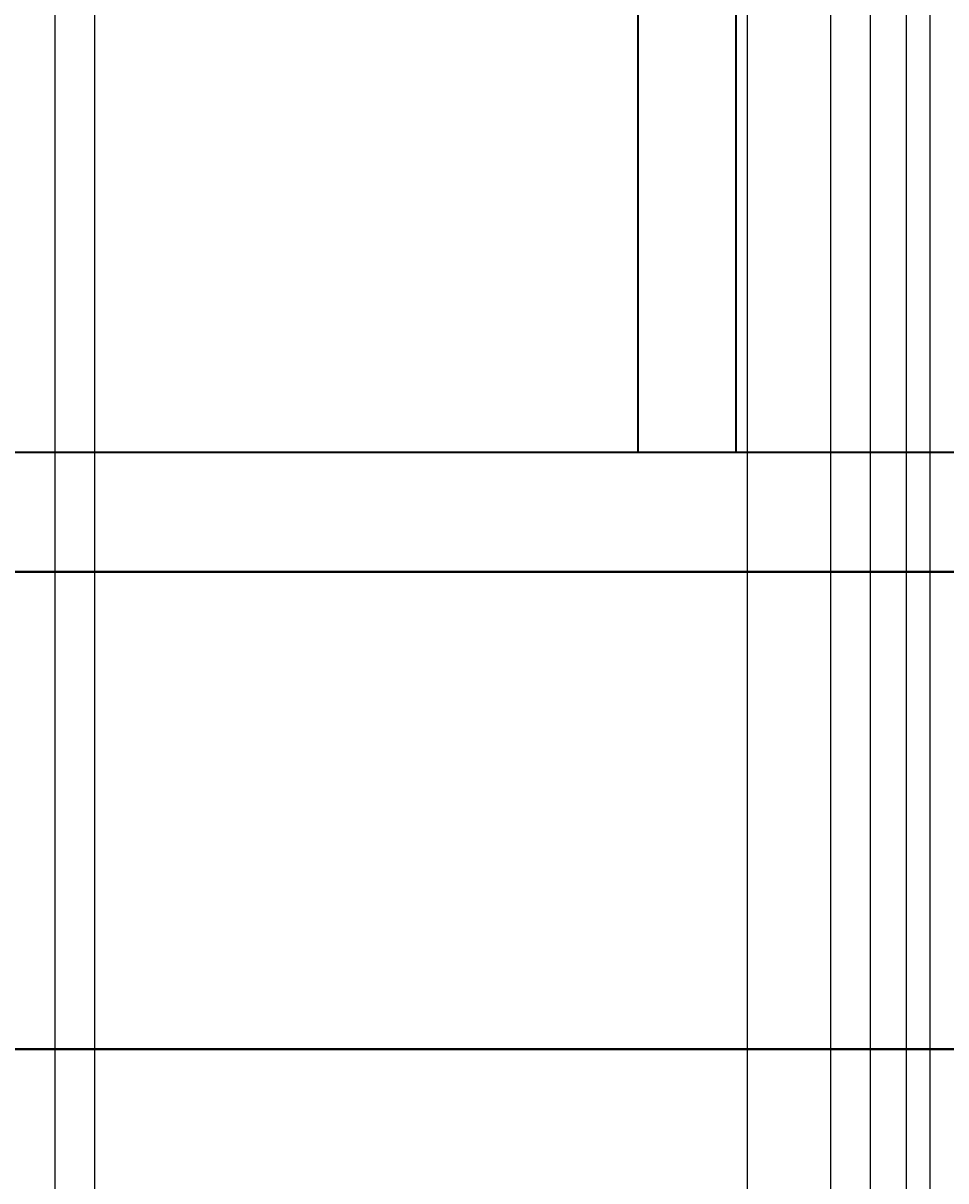
# Model space of a CAD drawing. Units: inches. Extents: x -6 to 289, y -8 to 323.
# Tile 52 of 107: x 146 to 169, y 124 to 153. Entities that reach past the tile are written whole.
import ezdxf

# ---------------------------------------------------------------- set-up
doc = ezdxf.new("R2010")
doc.units = ezdxf.units.IN
doc.header["$MEASUREMENT"] = 0
doc.layers.add('A-ANNO-DIMS', color=2, linetype='Continuous', lineweight=18)
doc.layers.add('A-ELEV', color=7, linetype='Continuous', lineweight=35)
doc.styles.get("Standard").update_dxf_attribs({"font": 'arial.ttf'})
doc.dimstyles.get("Standard").update_dxf_attribs({"dimtxt": 0.18, "dimasz": 0.18, "dimexe": 0.18, "dimexo": 0.0625, "dimgap": 0.09, "dimtad": 0, "dimtih": 1, "dimtoh": 1, "dimdec": 4, "dimzin": 0, "dimdsep": 46, "dimtxsty": 'Standard', "dimcen": 0.09, "dimadec": 0, "dimazin": 0, "dimtfac": 1, "dimtdec": 4, "dimtofl": 0, "dimtmove": 0, "dimatfit": 3, "dimfxl": 1, "dimtolj": 1, "dimtzin": 0, "dimarcsym": 0})

# ---------------------------------------------------------------- blocks, each defined once
blk = doc.blocks.new('*D24')
at = {"layer": 'A-ANNO-DIMS', "color": 0, "lineweight": -2, "transparency": 16777216}
for p, q in [((126.946, 178.654), (288.653, 178.654)), ((288.473, 178.474), (288.473, 159.153)), ((288.473, 139.469), (288.473, 158.789)), ((259.226, 139.289), (288.653, 139.289))]:
    blk.add_line(p, q, dxfattribs=at)
at = {"layer": 'A-ANNO-DIMS', "color": 0, "transparency": 16777216}
for points in [[(288.443, 178.474), (288.503, 178.474), (288.473, 178.654)], [(288.443, 139.469), (288.503, 139.469), (288.473, 139.289)]]:
    blk.add_solid(points, dxfattribs=at)
at = {"layer": 'Defpoints', "color": 0, "transparency": 16777216}
for p in [(126.883, 178.654), (288.473, 178.654), (259.164, 139.289)]:
    blk.add_point(p, dxfattribs=at)
at = {"layer": 'A-ANNO-DIMS', "color": 0, "transparency": 16777216, "insert": (288.473, 158.971), "char_height": 0.18, "attachment_point": 5}
blk.add_mtext('\\A1;39.365', dxfattribs=at)
blk = doc.blocks.new('*D30')
at = {"layer": 'A-ANNO-DIMS', "color": 0, "lineweight": -2, "transparency": 16777216}
for p, q in [((129.383, 181.092), (129.383, -8.391)), ((146.883, 181.092), (146.883, -8.391)), ((129.563, -8.211), (137.817, -8.211)), ((146.703, -8.211), (138.449, -8.211))]:
    blk.add_line(p, q, dxfattribs=at)
at = {"layer": 'A-ANNO-DIMS', "color": 0, "transparency": 16777216}
for points in [[(129.563, -8.181), (129.563, -8.241), (129.383, -8.211)], [(146.703, -8.181), (146.703, -8.241), (146.883, -8.211)]]:
    blk.add_solid(points, dxfattribs=at)
at = {"layer": 'Defpoints', "color": 0, "transparency": 16777216}
for p in [(129.383, 181.154), (146.883, 181.154), (146.883, -8.211)]:
    blk.add_point(p, dxfattribs=at)
at = {"layer": 'A-ANNO-DIMS', "color": 0, "transparency": 16777216, "insert": (138.133, -8.211), "char_height": 0.18, "attachment_point": 5}
blk.add_mtext('\\A1;17.5', dxfattribs=at)
blk = doc.blocks.new('*D31')
at = {"layer": 'A-ANNO-DIMS', "color": 0, "lineweight": -2, "transparency": 16777216}
for p, q in [((146.883, 181.092), (146.883, -8.391)), ((147.883, 181.092), (147.883, -8.391)), ((147.063, -8.211), (147.26, -8.211)), ((147.703, -8.211), (147.507, -8.211))]:
    blk.add_line(p, q, dxfattribs=at)
at = {"layer": 'A-ANNO-DIMS', "color": 0, "transparency": 16777216}
for points in [[(147.063, -8.181), (147.063, -8.241), (146.883, -8.211)], [(147.703, -8.181), (147.703, -8.241), (147.883, -8.211)]]:
    blk.add_solid(points, dxfattribs=at)
at = {"layer": 'Defpoints', "color": 0, "transparency": 16777216}
for p in [(146.883, 181.154), (147.883, 181.154), (147.883, -8.211)]:
    blk.add_point(p, dxfattribs=at)
at = {"layer": 'A-ANNO-DIMS', "color": 0, "transparency": 16777216, "insert": (147.383, -8.211), "char_height": 0.18, "attachment_point": 5}
blk.add_mtext('\\A1;1', dxfattribs=at)
blk = doc.blocks.new('*D32')
at = {"layer": 'A-ANNO-DIMS', "color": 0, "lineweight": -2, "transparency": 16777216}
for p, q in [((147.883, 181.092), (147.883, -8.391)), ((166.383, 181.092), (166.383, -8.391)), ((148.063, -8.211), (156.817, -8.211)), ((166.203, -8.211), (157.449, -8.211))]:
    blk.add_line(p, q, dxfattribs=at)
at = {"layer": 'A-ANNO-DIMS', "color": 0, "transparency": 16777216}
for points in [[(148.063, -8.181), (148.063, -8.241), (147.883, -8.211)], [(166.203, -8.181), (166.203, -8.241), (166.383, -8.211)]]:
    blk.add_solid(points, dxfattribs=at)
at = {"layer": 'Defpoints', "color": 0, "transparency": 16777216}
for p in [(147.883, 181.154), (166.383, 181.154), (166.383, -8.211)]:
    blk.add_point(p, dxfattribs=at)
at = {"layer": 'A-ANNO-DIMS', "color": 0, "transparency": 16777216, "insert": (157.133, -8.211), "char_height": 0.18, "attachment_point": 5}
blk.add_mtext('\\A1;18.5', dxfattribs=at)
blk = doc.blocks.new('*D33')
at = {"layer": 'A-ANNO-DIMS', "color": 0, "lineweight": -2, "transparency": 16777216}
for p, q in [((166.383, 181.092), (166.383, -8.391)), ((167.383, 180.092), (167.383, -8.391)), ((166.563, -8.211), (166.76, -8.211)), ((167.203, -8.211), (167.007, -8.211))]:
    blk.add_line(p, q, dxfattribs=at)
at = {"layer": 'A-ANNO-DIMS', "color": 0, "transparency": 16777216}
for points in [[(166.563, -8.181), (166.563, -8.241), (166.383, -8.211)], [(167.203, -8.181), (167.203, -8.241), (167.383, -8.211)]]:
    blk.add_solid(points, dxfattribs=at)
at = {"layer": 'Defpoints', "color": 0, "transparency": 16777216}
for p in [(166.383, 181.154), (167.383, 180.154), (167.383, -8.211)]:
    blk.add_point(p, dxfattribs=at)
at = {"layer": 'A-ANNO-DIMS', "color": 0, "transparency": 16777216, "insert": (166.883, -8.211), "char_height": 0.18, "attachment_point": 5}
blk.add_mtext('\\A1;1', dxfattribs=at)
blk = doc.blocks.new('*D34')
at = {"layer": 'A-ANNO-DIMS', "color": 0, "lineweight": -2, "transparency": 16777216}
for p, q in [((167.383, 180.092), (167.383, -8.391)), ((168.883, 178.592), (168.883, -8.391)), ((167.563, -8.211), (167.887, -8.211)), ((168.703, -8.211), (168.38, -8.211))]:
    blk.add_line(p, q, dxfattribs=at)
at = {"layer": 'A-ANNO-DIMS', "color": 0, "transparency": 16777216}
for points in [[(167.563, -8.181), (167.563, -8.241), (167.383, -8.211)], [(168.703, -8.181), (168.703, -8.241), (168.883, -8.211)]]:
    blk.add_solid(points, dxfattribs=at)
at = {"layer": 'Defpoints', "color": 0, "transparency": 16777216}
for p in [(167.383, 180.154), (168.883, 178.654), (168.883, -8.211)]:
    blk.add_point(p, dxfattribs=at)
at = {"layer": 'A-ANNO-DIMS', "color": 0, "transparency": 16777216, "insert": (168.133, -8.211), "char_height": 0.18, "attachment_point": 5}
blk.add_mtext('\\A1;1.5', dxfattribs=at)
blk = doc.blocks.new('*D76')
at = {"layer": 'A-ANNO-DIMS', "color": 0, "lineweight": -2, "transparency": 16777216}
for p, q in [((142.296, 51.148), (142.296, 322.969)), ((164.296, 51.148), (164.296, 322.969)), ((142.476, 322.789), (153.076, 322.789)), ((164.116, 322.789), (153.516, 322.789))]:
    blk.add_line(p, q, dxfattribs=at)
at = {"layer": 'A-ANNO-DIMS', "color": 0, "transparency": 16777216}
for points in [[(142.476, 322.819), (142.476, 322.759), (142.296, 322.789)], [(164.116, 322.819), (164.116, 322.759), (164.296, 322.789)]]:
    blk.add_solid(points, dxfattribs=at)
at = {"layer": 'Defpoints', "color": 0, "transparency": 16777216}
for p in [(164.296, 322.789), (142.296, 51.085), (164.296, 51.085)]:
    blk.add_point(p, dxfattribs=at)
at = {"layer": 'A-ANNO-DIMS', "color": 0, "transparency": 16777216, "insert": (153.296, 322.789), "char_height": 0.18, "attachment_point": 5}
blk.add_mtext('\\A1;22', dxfattribs=at)
blk = doc.blocks.new('*D77')
at = {"layer": 'A-ANNO-DIMS', "color": 0, "lineweight": -2, "transparency": 16777216}
for p, q in [((164.296, 51.148), (164.296, 322.969)), ((168.296, 51.148), (168.296, 322.969)), ((164.476, 322.789), (166.144, 322.789)), ((168.116, 322.789), (166.448, 322.789))]:
    blk.add_line(p, q, dxfattribs=at)
at = {"layer": 'A-ANNO-DIMS', "color": 0, "transparency": 16777216}
for points in [[(164.476, 322.819), (164.476, 322.759), (164.296, 322.789)], [(168.116, 322.819), (168.116, 322.759), (168.296, 322.789)]]:
    blk.add_solid(points, dxfattribs=at)
at = {"layer": 'Defpoints', "color": 0, "transparency": 16777216}
for p in [(168.296, 322.789), (164.296, 51.085), (168.296, 51.085)]:
    blk.add_point(p, dxfattribs=at)
at = {"layer": 'A-ANNO-DIMS', "color": 0, "transparency": 16777216, "insert": (166.296, 322.789), "char_height": 0.18, "attachment_point": 5}
blk.add_mtext('\\A1;4', dxfattribs=at)
blk = doc.blocks.new('*D78')
at = {"layer": 'A-ANNO-DIMS', "color": 0, "lineweight": -2, "transparency": 16777216}
for p, q in [((168.296, 51.148), (168.296, 322.969)), ((171.296, 51.148), (171.296, 322.969)), ((168.476, 322.789), (169.647, 322.789)), ((171.116, 322.789), (169.945, 322.789))]:
    blk.add_line(p, q, dxfattribs=at)
at = {"layer": 'A-ANNO-DIMS', "color": 0, "transparency": 16777216}
for points in [[(168.476, 322.819), (168.476, 322.759), (168.296, 322.789)], [(171.116, 322.819), (171.116, 322.759), (171.296, 322.789)]]:
    blk.add_solid(points, dxfattribs=at)
at = {"layer": 'Defpoints', "color": 0, "transparency": 16777216}
for p in [(171.296, 322.789), (168.296, 51.085), (171.296, 51.085)]:
    blk.add_point(p, dxfattribs=at)
at = {"layer": 'A-ANNO-DIMS', "color": 0, "transparency": 16777216, "insert": (169.796, 322.789), "char_height": 0.18, "attachment_point": 5}
blk.add_mtext('\\A1;3', dxfattribs=at)

msp = doc.modelspace()

# ---------------------------------------------------------------- linework, layer by layer
at = {"layer": 'A-ELEV'}
for p, q in [((115.1638, 139.2888), (259.1638, 139.2888)), ((259.1638, 127.2888), (115.1638, 127.2888)), ((115.1638, 127.2888), (259.1638, 127.2888))]:
    msp.add_line(p, q, dxfattribs=at)
for points in [[(247.1638, 139.2888), (115.1638, 139.2888), (115.1638, 162.3484), (247.1638, 162.3484)], [(244.1638, 142.2888), (118.1638, 142.2888), (118.1638, 159.3484), (244.1638, 159.3484)], [(161.5522, 159.3484), (164.0039, 159.3484), (164.0039, 142.2888), (161.5522, 142.2888)]]:
    msp.add_lwpolyline(points, close=True, dxfattribs=at)

# ---------------------------------------------------------------- dimensions: what is measured, and where the dimension line sits
at = {"layer": 'A-ANNO-DIMS'}
for base, p1, p2, override, picture, middle in [((164.296, 322.7888), (142.296, 51.0851), (164.296, 51.0851), {"dimdec": 0, "dimlfac": 1, "dimrnd": 0, "dimzin": 0, "dimdsep": 46, "dimlunit": 2}, '*D76', (153.296, 322.7888)), ((168.296, 322.7888), (164.296, 51.0851), (168.296, 51.0851), {"dimdec": 0, "dimlfac": 1, "dimrnd": 0, "dimzin": 0, "dimdsep": 46, "dimlunit": 2}, '*D77', (166.296, 322.7888)), ((171.296, 322.7888), (168.296, 51.0851), (171.296, 51.0851), {"dimdec": 0, "dimlfac": 1, "dimrnd": 0, "dimzin": 0, "dimdsep": 46, "dimlunit": 2}, '*D78', (169.796, 322.7888)), ((146.8835, -8.2112), (129.3835, 181.154), (146.8835, 181.154), {"dimdec": 1, "dimlfac": 1, "dimrnd": 0, "dimzin": 0, "dimdsep": 46, "dimlunit": 2}, '*D30', (138.1335, -8.2112)), ((147.8835, -8.2112), (146.8835, 181.154), (147.8835, 181.154), {"dimdec": 0, "dimlfac": 1, "dimrnd": 0, "dimzin": 0, "dimdsep": 46, "dimlunit": 2}, '*D31', (147.3835, -8.2112)), ((166.3835, -8.2112), (147.8835, 181.154), (166.3835, 181.154), {"dimdec": 1, "dimlfac": 1, "dimrnd": 0, "dimzin": 0, "dimdsep": 46, "dimlunit": 2}, '*D32', (157.1335, -8.2112)), ((167.3835, -8.2112), (166.3835, 181.154), (167.3835, 180.154), {"dimdec": 0, "dimlfac": 1, "dimrnd": 0, "dimzin": 0, "dimdsep": 46, "dimlunit": 2}, '*D33', (166.8835, -8.2112)), ((168.8835, -8.2112), (167.3835, 180.154), (168.8835, 178.654), {"dimdec": 1, "dimlfac": 1, "dimrnd": 0, "dimzin": 0, "dimdsep": 46, "dimlunit": 2}, '*D34', (168.1335, -8.2112))]:
    dim = msp.add_linear_dim(base=base, p1=p1, p2=p2, dimstyle='Standard', override=override, dxfattribs=at)
    dim.commit()
    dim.dimension.update_dxf_attribs({"geometry": picture, "text_midpoint": middle})
dim = msp.add_linear_dim(base=(288.4733, 178.654), p1=(259.1638, 139.2888), p2=(126.8835, 178.654), angle=90, dimstyle='Standard', override={"dimdec": 3, "dimlfac": 1, "dimrnd": 0, "dimzin": 0, "dimdsep": 46, "dimlunit": 2}, dxfattribs=at)
dim.commit()
dim.dimension.update_dxf_attribs({"geometry": '*D24', "text_midpoint": (288.4733, 158.9714)})

doc.saveas('drawing.dxf')
